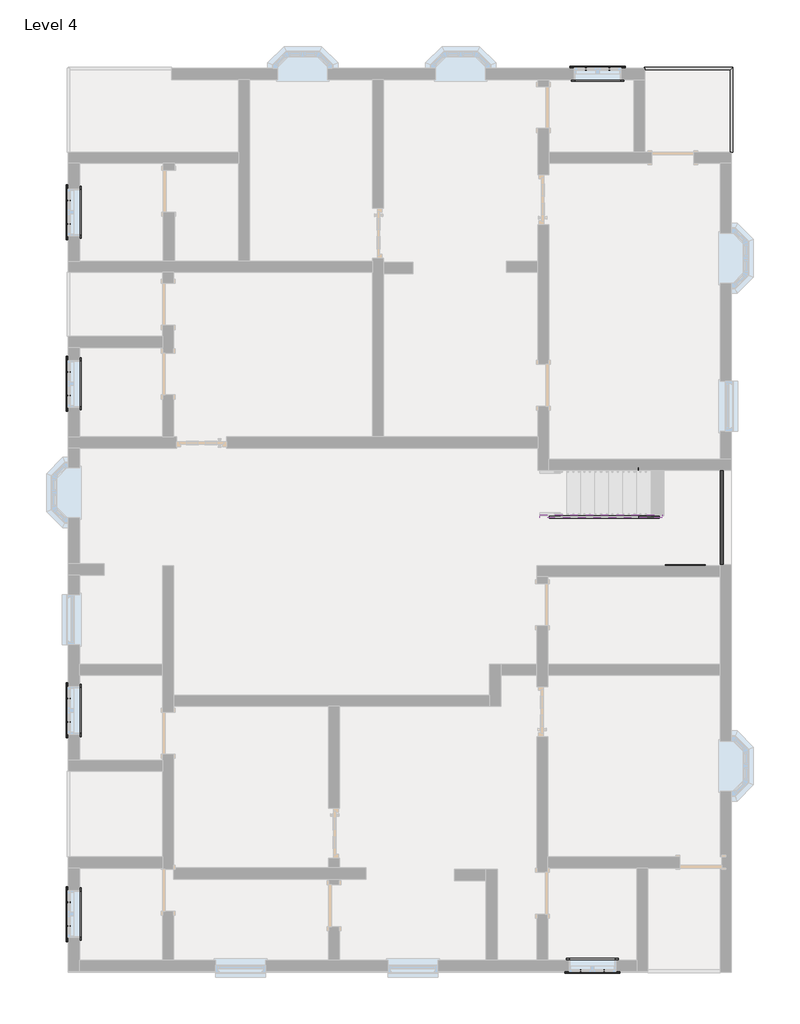
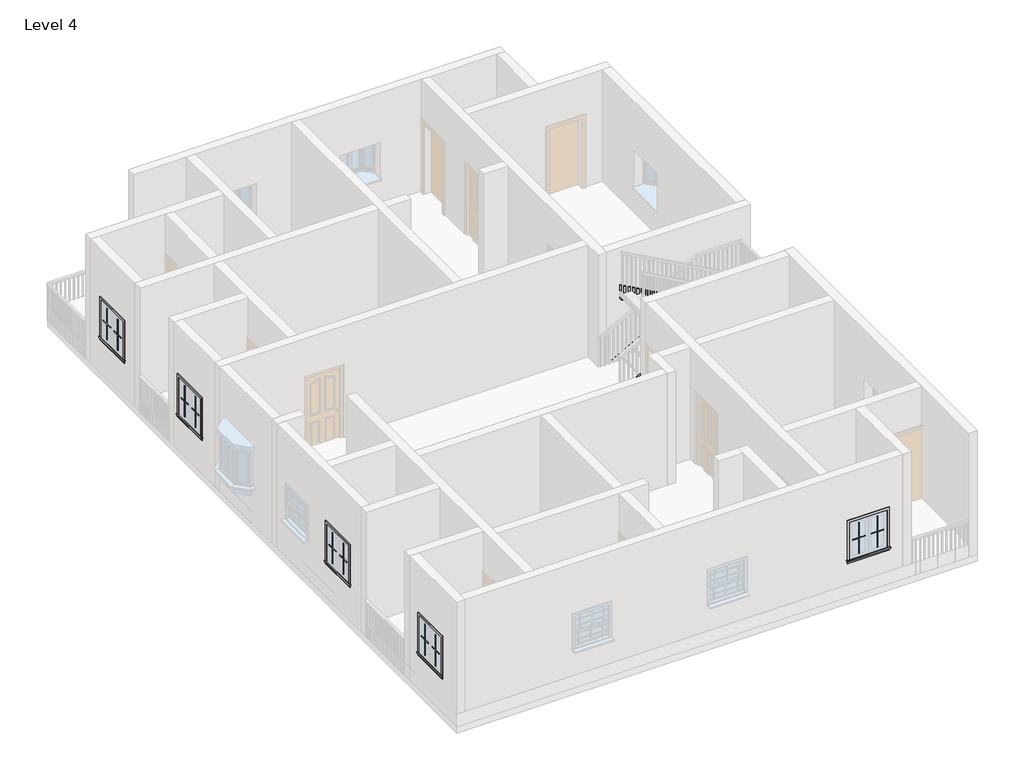
# One storey, part 4 of 4: 24 proxies, 5 members, 1 railing.
"""IFC4 building model written with IfcOpenShell, lengths in millimetres."""

from ifc_helpers import new_model, si_unit, frame, origin, place, context, project, spatial, polyline, outline, extrude, faceted_brep, transform, mapped, element, save
from components import muntin_pattern_2x2_muntin_pattern_2x2_b3fe6957, muntin_pattern_2x2_muntin_pattern_2x2_3e0ecaf2, trim_window_exterior_flat_with_sill_41619996, trim_window_interior_flat_picture_frame_51c85655

model = new_model("IFC4")

# Units and contexts
model_context = context("Model", 3, world=origin())
ifc_project = project(units=[si_unit("LENGTHUNIT", "METRE", prefix="MILLI")], contexts=[model_context])

# Site, building, storey
site = spatial("IfcSite", under=ifc_project)
building = spatial("IfcBuilding", under=site)
storey = spatial("IfcBuildingStorey", under=building, Name="Level 4", Elevation=9144.0)

# Proxies
placement = place(None, origin())
muntin_pattern_2x2_muntin_pattern_2x2_shape = muntin_pattern_2x2_muntin_pattern_2x2_b3fe6957(model_context)
element("IfcBuildingElementProxy", 1, Name="Muntin Pattern_2x2 : Muntin Pattern_2x2", ObjectType="Muntin Pattern_2x2 : Muntin Pattern_2x2", at=placement, inside=storey, context=model_context, shape_type="MappedRepresentation", body=[
    mapped(muntin_pattern_2x2_muntin_pattern_2x2_shape, transform((-7038.4808717, 5489.0318597, 10128.25), x_axis=(0.0, 1.0, 0.0), y_axis=(-1.0, 0.0, 0.0), z_axis=(0.0, 0.0, 1.0))),
])
element("IfcBuildingElementProxy", 2, Name="Muntin Pattern_2x2 : Muntin Pattern_2x2", ObjectType="Muntin Pattern_2x2 : Muntin Pattern_2x2", at=placement, inside=storey, context=model_context, shape_type="MappedRepresentation", body=[
    mapped(muntin_pattern_2x2_muntin_pattern_2x2_shape, transform((-7038.4808717, 2366.9422293, 10128.25), x_axis=(0.0, 1.0, 0.0), y_axis=(-1.0, 0.0, 0.0), z_axis=(0.0, 0.0, 1.0))),
])
element("IfcBuildingElementProxy", 3, Name="Muntin Pattern_2x2 : Muntin Pattern_2x2", ObjectType="Muntin Pattern_2x2 : Muntin Pattern_2x2", at=placement, inside=storey, context=model_context, shape_type="MappedRepresentation", body=[
    mapped(muntin_pattern_2x2_muntin_pattern_2x2_shape, transform((2376.9816283, 8312.1297293, 10128.25), x_axis=(1.0, 0.0, 0.0), y_axis=(0.0, 1.0, 0.0), z_axis=(0.0, 0.0, 1.0))),
])
element("IfcBuildingElementProxy", 4, Name="Muntin Pattern_2x2 : Muntin Pattern_2x2", ObjectType="Muntin Pattern_2x2 : Muntin Pattern_2x2", at=placement, inside=storey, context=model_context, shape_type="MappedRepresentation", body=[
    mapped(muntin_pattern_2x2_muntin_pattern_2x2_shape, transform((2710.3566283, -8102.6202707, 10128.25), x_axis=(-1.0, 0.0, 0.0), y_axis=(0.0, -1.0, 0.0), z_axis=(0.0, 0.0, 1.0))),
])
element("IfcBuildingElementProxy", 5, Name="Muntin Pattern_2x2 : Muntin Pattern_2x2", ObjectType="Muntin Pattern_2x2 : Muntin Pattern_2x2", at=placement, inside=storey, context=model_context, shape_type="MappedRepresentation", body=[
    mapped(muntin_pattern_2x2_muntin_pattern_2x2_shape, transform((-7038.4808717, -7285.0577707, 10128.25), x_axis=(0.0, 1.0, 0.0), y_axis=(-1.0, 0.0, 0.0), z_axis=(0.0, 0.0, 1.0))),
])
element("IfcBuildingElementProxy", 6, Name="Muntin Pattern_2x2 : Muntin Pattern_2x2", ObjectType="Muntin Pattern_2x2 : Muntin Pattern_2x2", at=placement, inside=storey, context=model_context, shape_type="MappedRepresentation", body=[
    mapped(muntin_pattern_2x2_muntin_pattern_2x2_shape, transform((-7038.4808717, -3576.6577707, 10128.25), x_axis=(0.0, 1.0, 0.0), y_axis=(-1.0, 0.0, 0.0), z_axis=(0.0, 0.0, 1.0))),
])
muntin_pattern_2x2_muntin_pattern_2x2_2_shape = muntin_pattern_2x2_muntin_pattern_2x2_3e0ecaf2(model_context)
element("IfcBuildingElementProxy", 7, Name="Muntin Pattern_2x2 : Muntin Pattern_2x2", ObjectType="Muntin Pattern_2x2 : Muntin Pattern_2x2", at=placement, inside=storey, context=model_context, shape_type="MappedRepresentation", body=[
    mapped(muntin_pattern_2x2_muntin_pattern_2x2_2_shape, transform((-7038.4808717, 5917.6568597, 10128.25), x_axis=(0.0, -1.0, 0.0), y_axis=(1.0, 0.0, 0.0), z_axis=(0.0, 0.0, 1.0))),
])
element("IfcBuildingElementProxy", 8, Name="Muntin Pattern_2x2 : Muntin Pattern_2x2", ObjectType="Muntin Pattern_2x2 : Muntin Pattern_2x2", at=placement, inside=storey, context=model_context, shape_type="MappedRepresentation", body=[
    mapped(muntin_pattern_2x2_muntin_pattern_2x2_2_shape, transform((-7038.4808717, 2795.5672293, 10128.25), x_axis=(0.0, -1.0, 0.0), y_axis=(1.0, 0.0, 0.0), z_axis=(0.0, 0.0, 1.0))),
])
element("IfcBuildingElementProxy", 9, Name="Muntin Pattern_2x2 : Muntin Pattern_2x2", ObjectType="Muntin Pattern_2x2 : Muntin Pattern_2x2", at=placement, inside=storey, context=model_context, shape_type="MappedRepresentation", body=[
    mapped(muntin_pattern_2x2_muntin_pattern_2x2_2_shape, transform((2805.6066283, 8312.1297293, 10128.25), x_axis=(-1.0, 0.0, 0.0), y_axis=(0.0, -1.0, 0.0), z_axis=(0.0, 0.0, 1.0))),
])
element("IfcBuildingElementProxy", 10, Name="Muntin Pattern_2x2 : Muntin Pattern_2x2", ObjectType="Muntin Pattern_2x2 : Muntin Pattern_2x2", at=placement, inside=storey, context=model_context, shape_type="MappedRepresentation", body=[
    mapped(muntin_pattern_2x2_muntin_pattern_2x2_2_shape, transform((2281.7316283, -8102.6202707, 10128.25), x_axis=(1.0, 0.0, 0.0), y_axis=(0.0, 1.0, 0.0), z_axis=(0.0, 0.0, 1.0))),
])
element("IfcBuildingElementProxy", 11, Name="Muntin Pattern_2x2 : Muntin Pattern_2x2", ObjectType="Muntin Pattern_2x2 : Muntin Pattern_2x2", at=placement, inside=storey, context=model_context, shape_type="MappedRepresentation", body=[
    mapped(muntin_pattern_2x2_muntin_pattern_2x2_2_shape, transform((-7038.4808717, -6856.4327707, 10128.25), x_axis=(0.0, -1.0, 0.0), y_axis=(1.0, 0.0, 0.0), z_axis=(0.0, 0.0, 1.0))),
])
element("IfcBuildingElementProxy", 12, Name="Muntin Pattern_2x2 : Muntin Pattern_2x2", ObjectType="Muntin Pattern_2x2 : Muntin Pattern_2x2", at=placement, inside=storey, context=model_context, shape_type="MappedRepresentation", body=[
    mapped(muntin_pattern_2x2_muntin_pattern_2x2_2_shape, transform((-7038.4808717, -3148.0327707, 10128.25), x_axis=(0.0, -1.0, 0.0), y_axis=(1.0, 0.0, 0.0), z_axis=(0.0, 0.0, 1.0))),
])
trim_window_exterior_flat_with_sill_shape = trim_window_exterior_flat_with_sill_41619996(model_context)
element("IfcBuildingElementProxy", 13, Name="Trim-Window-Exterior-Flat : with Sill", ObjectType="Trim-Window-Exterior-Flat : with Sill", at=placement, inside=storey, context=model_context, shape_type="MappedRepresentation", body=[
    mapped(trim_window_exterior_flat_with_sill_shape, transform((-7048.0058717, 5703.3443597, 10972.8), x_axis=(0.0, -1.0, 0.0), y_axis=(0.0, 0.0, 1.0), z_axis=(-1.0, 0.0, 0.0))),
])
element("IfcBuildingElementProxy", 14, Name="Trim-Window-Exterior-Flat : with Sill", ObjectType="Trim-Window-Exterior-Flat : with Sill", at=placement, inside=storey, context=model_context, shape_type="MappedRepresentation", body=[
    mapped(trim_window_exterior_flat_with_sill_shape, transform((-7048.0058717, 2581.2547293, 10972.8), x_axis=(0.0, -1.0, 0.0), y_axis=(0.0, 0.0, 1.0), z_axis=(-1.0, 0.0, 0.0))),
])
element("IfcBuildingElementProxy", 15, Name="Trim-Window-Exterior-Flat : with Sill", ObjectType="Trim-Window-Exterior-Flat : with Sill", at=placement, inside=storey, context=model_context, shape_type="MappedRepresentation", body=[
    mapped(trim_window_exterior_flat_with_sill_shape, transform((2591.2941283, 8321.6547293, 10972.8), x_axis=(-1.0, 0.0, 0.0), y_axis=(0.0, 0.0, 1.0), z_axis=(0.0, 1.0, 0.0))),
])
element("IfcBuildingElementProxy", 16, Name="Trim-Window-Exterior-Flat : with Sill", ObjectType="Trim-Window-Exterior-Flat : with Sill", at=placement, inside=storey, context=model_context, shape_type="MappedRepresentation", body=[
    mapped(trim_window_exterior_flat_with_sill_shape, transform((2496.0441283, -8112.1452707, 10972.8), x_axis=(1.0, 0.0, 0.0), y_axis=(0.0, 0.0, 1.0), z_axis=(0.0, -1.0, 0.0))),
])
element("IfcBuildingElementProxy", 17, Name="Trim-Window-Exterior-Flat : with Sill", ObjectType="Trim-Window-Exterior-Flat : with Sill", at=placement, inside=storey, context=model_context, shape_type="MappedRepresentation", body=[
    mapped(trim_window_exterior_flat_with_sill_shape, transform((-7048.0058717, -7070.7452707, 10972.8), x_axis=(0.0, -1.0, 0.0), y_axis=(0.0, 0.0, 1.0), z_axis=(-1.0, 0.0, 0.0))),
])
element("IfcBuildingElementProxy", 18, Name="Trim-Window-Exterior-Flat : with Sill", ObjectType="Trim-Window-Exterior-Flat : with Sill", at=placement, inside=storey, context=model_context, shape_type="MappedRepresentation", body=[
    mapped(trim_window_exterior_flat_with_sill_shape, transform((-7048.0058717, -3362.3452707, 10972.8), x_axis=(0.0, -1.0, 0.0), y_axis=(0.0, 0.0, 1.0), z_axis=(-1.0, 0.0, 0.0))),
])
trim_window_interior_flat_picture_frame_shape = trim_window_interior_flat_picture_frame_51c85655(model_context)
element("IfcBuildingElementProxy", 19, Name="Trim-Window-Interior-Flat : Picture Frame", ObjectType="Trim-Window-Interior-Flat : Picture Frame", at=placement, inside=storey, context=model_context, shape_type="MappedRepresentation", body=[
    mapped(trim_window_interior_flat_picture_frame_shape, transform((-6844.8058717, 5703.3443597, 10972.8), x_axis=(0.0, 1.0, 0.0), y_axis=(0.0, 0.0, 1.0), z_axis=(1.0, 0.0, 0.0))),
])
element("IfcBuildingElementProxy", 20, Name="Trim-Window-Interior-Flat : Picture Frame", ObjectType="Trim-Window-Interior-Flat : Picture Frame", at=placement, inside=storey, context=model_context, shape_type="MappedRepresentation", body=[
    mapped(trim_window_interior_flat_picture_frame_shape, transform((-6844.8058717, 2581.2547293, 10972.8), x_axis=(0.0, 1.0, 0.0), y_axis=(0.0, 0.0, 1.0), z_axis=(1.0, 0.0, 0.0))),
])
element("IfcBuildingElementProxy", 21, Name="Trim-Window-Interior-Flat : Picture Frame", ObjectType="Trim-Window-Interior-Flat : Picture Frame", at=placement, inside=storey, context=model_context, shape_type="MappedRepresentation", body=[
    mapped(trim_window_interior_flat_picture_frame_shape, transform((2591.2941283, 8118.4547293, 10972.8), x_axis=(1.0, 0.0, 0.0), y_axis=(0.0, 0.0, 1.0), z_axis=(0.0, -1.0, 0.0))),
])
element("IfcBuildingElementProxy", 22, Name="Trim-Window-Interior-Flat : Picture Frame", ObjectType="Trim-Window-Interior-Flat : Picture Frame", at=placement, inside=storey, context=model_context, shape_type="MappedRepresentation", body=[
    mapped(trim_window_interior_flat_picture_frame_shape, transform((2496.0441283, -7908.9452707, 10972.8), x_axis=(-1.0, 0.0, 0.0), y_axis=(0.0, 0.0, 1.0), z_axis=(0.0, 1.0, 0.0))),
])
element("IfcBuildingElementProxy", 23, Name="Trim-Window-Interior-Flat : Picture Frame", ObjectType="Trim-Window-Interior-Flat : Picture Frame", at=placement, inside=storey, context=model_context, shape_type="MappedRepresentation", body=[
    mapped(trim_window_interior_flat_picture_frame_shape, transform((-6844.8058717, -7070.7452707, 10972.8), x_axis=(0.0, 1.0, 0.0), y_axis=(0.0, 0.0, 1.0), z_axis=(1.0, 0.0, 0.0))),
])
element("IfcBuildingElementProxy", 24, Name="Trim-Window-Interior-Flat : Picture Frame", ObjectType="Trim-Window-Interior-Flat : Picture Frame", at=placement, inside=storey, context=model_context, shape_type="MappedRepresentation", body=[
    mapped(trim_window_interior_flat_picture_frame_shape, transform((-6844.8058717, -3362.3452707, 10972.8), x_axis=(0.0, 1.0, 0.0), y_axis=(0.0, 0.0, 1.0), z_axis=(1.0, 0.0, 0.0))),
])

# Members
element("IfcMember", 25, ObjectType="Stringer - 2\" Width", at=placement, inside=storey, context=model_context, shape_type="SweptSolid", body=[
    extrude(outline(polyline([(9354.6757607, 1537.1941283), (9144.0, 1537.1941283), (9144.0, 1786.1766781), (10591.8, 4407.1563102), (10591.8, 3776.7834593), (9354.6757607, 1537.1941283)])), frame((0.0, 1006.4547293, 0.0), z_axis=(0.0, 1.0, 0.0), x_axis=(0.0, 0.0, 1.0)), (0.0, 0.0, 1.0), 50.8),
])
element("IfcMember", 26, ObjectType="Stringer - 2\" Width", at=placement, inside=storey, context=model_context, shape_type="SweptSolid", body=[
    extrude(outline(polyline([(4826.4941283, 1057.2547293), (4877.2941283, 1057.2547293), (4877.2941283, -714.2964201), (4826.4941283, -714.2964201), (4826.4941283, 1057.2547293)])), frame((0.0, 0.0, 10287.0), z_axis=(0.0, 0.0, 1.0), x_axis=(1.0, 0.0, 0.0)), (0.0, 0.0, 1.0), 304.8),
])
element("IfcMember", 27, ObjectType="Stringer - 2\" Width", at=placement, inside=storey, context=model_context, shape_type="SweptSolid", body=[
    extrude(outline(polyline([(10287.0, 4555.0346706), (11954.0215532, 1537.1941283), (11605.8106009, 1537.1941283), (10287.0, 3924.6618197), (10287.0, 4555.0346706)])), frame((0.0, -765.0964201, 0.0), z_axis=(0.0, 1.0, 0.0), x_axis=(0.0, 0.0, 1.0)), (0.0, 0.0, 1.0), 50.8),
])
element("IfcMember", 28, ObjectType="Stringer - 2\" Width", at=placement, inside=storey, context=model_context, shape_type="SweptSolid", body=[
    extrude(outline(polyline([(9354.6757607, 1537.1941283), (9144.0, 1537.1941283), (9144.0, 1786.1766781), (10209.4963497, 3715.0648053), (10557.7073019, 3715.0648053), (9354.6757607, 1537.1941283)])), frame((0.0, 130.1547293, 0.0), z_axis=(0.0, 1.0, 0.0), x_axis=(0.0, 0.0, 1.0)), (0.0, 0.0, 1.0), 50.8),
])
element("IfcMember", 29, ObjectType="Stringer - 2\" Width", at=placement, inside=storey, context=model_context, shape_type="SweptSolid", body=[
    extrude(outline(polyline([(10374.7177047, 3765.8648053), (10722.928657, 3765.8648053), (11954.0215532, 1537.1941283), (11605.8106009, 1537.1941283), (10374.7177047, 3765.8648053)])), frame((0.0, 142.8547293, 0.0), z_axis=(0.0, 1.0, 0.0), x_axis=(0.0, 0.0, 1.0)), (0.0, 0.0, 1.0), 50.8),
])

# Railing
element("IfcRailing", 30, ObjectType="Handrail - Rectangular", at=placement, inside=storey, context=model_context, shape_type="SolidModel", body=[
    faceted_brep([(3442.1941283, 8347.0547293, 10058.4), (3442.1941283, 8347.0547293, 10007.6), (3442.1941283, 8296.2547293, 10007.6), (3442.1941283, 8296.2547293, 10058.4), (5055.0941283, 8347.0547293, 10058.4), (5055.0941283, 8347.0547293, 10007.6), (5004.2941283, 8296.2547293, 10007.6), (5004.2941283, 8296.2547293, 10058.4), (5055.0941283, 6797.6547293, 10058.4), (5004.2941283, 6797.6547293, 10058.4), (5004.2941283, 6797.6547293, 10007.6), (5055.0941283, 6797.6547293, 10007.6)], [[[0, 1, 2, 3]], [[1, 0, 4, 5]], [[2, 1, 5, 6]], [[3, 2, 6, 7]], [[0, 3, 7, 4]], [[8, 9, 10, 11]], [[5, 4, 8, 11]], [[6, 5, 11, 10]], [[7, 6, 10, 9]], [[4, 7, 9, 8]]]),
    extrude(outline(polyline([(5020.1691283, 6908.7797293), (5039.2191283, 6908.7797293), (5039.2191283, 6889.7297293), (5020.1691283, 6889.7297293), (5020.1691283, 6908.7797293)])), frame((0.0, 0.0, 9144.0), z_axis=(0.0, 0.0, 1.0), x_axis=(1.0, 0.0, 0.0)), (0.0, 0.0, 1.0), 863.6),
    extrude(outline(polyline([(5020.1691283, 7010.3797293), (5039.2191283, 7010.3797293), (5039.2191283, 6991.3297293), (5020.1691283, 6991.3297293), (5020.1691283, 7010.3797293)])), frame((0.0, 0.0, 9144.0), z_axis=(0.0, 0.0, 1.0), x_axis=(1.0, 0.0, 0.0)), (0.0, 0.0, 1.0), 863.6),
    extrude(outline(polyline([(5020.1691283, 7111.9797293), (5039.2191283, 7111.9797293), (5039.2191283, 7092.9297293), (5020.1691283, 7092.9297293), (5020.1691283, 7111.9797293)])), frame((0.0, 0.0, 9144.0), z_axis=(0.0, 0.0, 1.0), x_axis=(1.0, 0.0, 0.0)), (0.0, 0.0, 1.0), 863.6),
    extrude(outline(polyline([(5020.1691283, 7213.5797293), (5039.2191283, 7213.5797293), (5039.2191283, 7194.5297293), (5020.1691283, 7194.5297293), (5020.1691283, 7213.5797293)])), frame((0.0, 0.0, 9144.0), z_axis=(0.0, 0.0, 1.0), x_axis=(1.0, 0.0, 0.0)), (0.0, 0.0, 1.0), 863.6),
    extrude(outline(polyline([(5020.1691283, 7315.1797293), (5039.2191283, 7315.1797293), (5039.2191283, 7296.1297293), (5020.1691283, 7296.1297293), (5020.1691283, 7315.1797293)])), frame((0.0, 0.0, 9144.0), z_axis=(0.0, 0.0, 1.0), x_axis=(1.0, 0.0, 0.0)), (0.0, 0.0, 1.0), 863.6),
    extrude(outline(polyline([(5020.1691283, 7416.7797293), (5039.2191283, 7416.7797293), (5039.2191283, 7397.7297293), (5020.1691283, 7397.7297293), (5020.1691283, 7416.7797293)])), frame((0.0, 0.0, 9144.0), z_axis=(0.0, 0.0, 1.0), x_axis=(1.0, 0.0, 0.0)), (0.0, 0.0, 1.0), 863.6),
    extrude(outline(polyline([(5020.1691283, 7518.3797293), (5039.2191283, 7518.3797293), (5039.2191283, 7499.3297293), (5020.1691283, 7499.3297293), (5020.1691283, 7518.3797293)])), frame((0.0, 0.0, 9144.0), z_axis=(0.0, 0.0, 1.0), x_axis=(1.0, 0.0, 0.0)), (0.0, 0.0, 1.0), 863.6),
    extrude(outline(polyline([(5020.1691283, 7619.9797293), (5039.2191283, 7619.9797293), (5039.2191283, 7600.9297293), (5020.1691283, 7600.9297293), (5020.1691283, 7619.9797293)])), frame((0.0, 0.0, 9144.0), z_axis=(0.0, 0.0, 1.0), x_axis=(1.0, 0.0, 0.0)), (0.0, 0.0, 1.0), 863.6),
    extrude(outline(polyline([(5020.1691283, 7721.5797293), (5039.2191283, 7721.5797293), (5039.2191283, 7702.5297293), (5020.1691283, 7702.5297293), (5020.1691283, 7721.5797293)])), frame((0.0, 0.0, 9144.0), z_axis=(0.0, 0.0, 1.0), x_axis=(1.0, 0.0, 0.0)), (0.0, 0.0, 1.0), 863.6),
    extrude(outline(polyline([(5020.1691283, 7823.1797293), (5039.2191283, 7823.1797293), (5039.2191283, 7804.1297293), (5020.1691283, 7804.1297293), (5020.1691283, 7823.1797293)])), frame((0.0, 0.0, 9144.0), z_axis=(0.0, 0.0, 1.0), x_axis=(1.0, 0.0, 0.0)), (0.0, 0.0, 1.0), 863.6),
    extrude(outline(polyline([(5020.1691283, 7924.7797293), (5039.2191283, 7924.7797293), (5039.2191283, 7905.7297293), (5020.1691283, 7905.7297293), (5020.1691283, 7924.7797293)])), frame((0.0, 0.0, 9144.0), z_axis=(0.0, 0.0, 1.0), x_axis=(1.0, 0.0, 0.0)), (0.0, 0.0, 1.0), 863.6),
    extrude(outline(polyline([(5020.1691283, 8026.3797293), (5039.2191283, 8026.3797293), (5039.2191283, 8007.3297293), (5020.1691283, 8007.3297293), (5020.1691283, 8026.3797293)])), frame((0.0, 0.0, 9144.0), z_axis=(0.0, 0.0, 1.0), x_axis=(1.0, 0.0, 0.0)), (0.0, 0.0, 1.0), 863.6),
    extrude(outline(polyline([(5020.1691283, 8127.9797293), (5039.2191283, 8127.9797293), (5039.2191283, 8108.9297293), (5020.1691283, 8108.9297293), (5020.1691283, 8127.9797293)])), frame((0.0, 0.0, 9144.0), z_axis=(0.0, 0.0, 1.0), x_axis=(1.0, 0.0, 0.0)), (0.0, 0.0, 1.0), 863.6),
    extrude(outline(polyline([(5020.1691283, 8229.5797293), (5039.2191283, 8229.5797293), (5039.2191283, 8210.5297293), (5020.1691283, 8210.5297293), (5020.1691283, 8229.5797293)])), frame((0.0, 0.0, 9144.0), z_axis=(0.0, 0.0, 1.0), x_axis=(1.0, 0.0, 0.0)), (0.0, 0.0, 1.0), 863.6),
    extrude(outline(polyline([(4956.6691283, 8312.1297293), (4956.6691283, 8331.1797293), (4975.7191283, 8331.1797293), (4975.7191283, 8312.1297293), (4956.6691283, 8312.1297293)])), frame((0.0, 0.0, 9144.0), z_axis=(0.0, 0.0, 1.0), x_axis=(1.0, 0.0, 0.0)), (0.0, 0.0, 1.0), 863.6),
    extrude(outline(polyline([(4855.0691283, 8312.1297293), (4855.0691283, 8331.1797293), (4874.1191283, 8331.1797293), (4874.1191283, 8312.1297293), (4855.0691283, 8312.1297293)])), frame((0.0, 0.0, 9144.0), z_axis=(0.0, 0.0, 1.0), x_axis=(1.0, 0.0, 0.0)), (0.0, 0.0, 1.0), 863.6),
    extrude(outline(polyline([(4753.4691283, 8312.1297293), (4753.4691283, 8331.1797293), (4772.5191283, 8331.1797293), (4772.5191283, 8312.1297293), (4753.4691283, 8312.1297293)])), frame((0.0, 0.0, 9144.0), z_axis=(0.0, 0.0, 1.0), x_axis=(1.0, 0.0, 0.0)), (0.0, 0.0, 1.0), 863.6),
    extrude(outline(polyline([(4651.8691283, 8312.1297293), (4651.8691283, 8331.1797293), (4670.9191283, 8331.1797293), (4670.9191283, 8312.1297293), (4651.8691283, 8312.1297293)])), frame((0.0, 0.0, 9144.0), z_axis=(0.0, 0.0, 1.0), x_axis=(1.0, 0.0, 0.0)), (0.0, 0.0, 1.0), 863.6),
    extrude(outline(polyline([(4550.2691283, 8312.1297293), (4550.2691283, 8331.1797293), (4569.3191283, 8331.1797293), (4569.3191283, 8312.1297293), (4550.2691283, 8312.1297293)])), frame((0.0, 0.0, 9144.0), z_axis=(0.0, 0.0, 1.0), x_axis=(1.0, 0.0, 0.0)), (0.0, 0.0, 1.0), 863.6),
    extrude(outline(polyline([(4448.6691283, 8312.1297293), (4448.6691283, 8331.1797293), (4467.7191283, 8331.1797293), (4467.7191283, 8312.1297293), (4448.6691283, 8312.1297293)])), frame((0.0, 0.0, 9144.0), z_axis=(0.0, 0.0, 1.0), x_axis=(1.0, 0.0, 0.0)), (0.0, 0.0, 1.0), 863.6),
    extrude(outline(polyline([(4347.0691283, 8312.1297293), (4347.0691283, 8331.1797293), (4366.1191283, 8331.1797293), (4366.1191283, 8312.1297293), (4347.0691283, 8312.1297293)])), frame((0.0, 0.0, 9144.0), z_axis=(0.0, 0.0, 1.0), x_axis=(1.0, 0.0, 0.0)), (0.0, 0.0, 1.0), 863.6),
    extrude(outline(polyline([(4245.4691283, 8312.1297293), (4245.4691283, 8331.1797293), (4264.5191283, 8331.1797293), (4264.5191283, 8312.1297293), (4245.4691283, 8312.1297293)])), frame((0.0, 0.0, 9144.0), z_axis=(0.0, 0.0, 1.0), x_axis=(1.0, 0.0, 0.0)), (0.0, 0.0, 1.0), 863.6),
    extrude(outline(polyline([(4143.8691283, 8312.1297293), (4143.8691283, 8331.1797293), (4162.9191283, 8331.1797293), (4162.9191283, 8312.1297293), (4143.8691283, 8312.1297293)])), frame((0.0, 0.0, 9144.0), z_axis=(0.0, 0.0, 1.0), x_axis=(1.0, 0.0, 0.0)), (0.0, 0.0, 1.0), 863.6),
    extrude(outline(polyline([(4042.2691283, 8312.1297293), (4042.2691283, 8331.1797293), (4061.3191283, 8331.1797293), (4061.3191283, 8312.1297293), (4042.2691283, 8312.1297293)])), frame((0.0, 0.0, 9144.0), z_axis=(0.0, 0.0, 1.0), x_axis=(1.0, 0.0, 0.0)), (0.0, 0.0, 1.0), 863.6),
    extrude(outline(polyline([(3940.6691283, 8312.1297293), (3940.6691283, 8331.1797293), (3959.7191283, 8331.1797293), (3959.7191283, 8312.1297293), (3940.6691283, 8312.1297293)])), frame((0.0, 0.0, 9144.0), z_axis=(0.0, 0.0, 1.0), x_axis=(1.0, 0.0, 0.0)), (0.0, 0.0, 1.0), 863.6),
    extrude(outline(polyline([(3839.0691283, 8312.1297293), (3839.0691283, 8331.1797293), (3858.1191283, 8331.1797293), (3858.1191283, 8312.1297293), (3839.0691283, 8312.1297293)])), frame((0.0, 0.0, 9144.0), z_axis=(0.0, 0.0, 1.0), x_axis=(1.0, 0.0, 0.0)), (0.0, 0.0, 1.0), 863.6),
    extrude(outline(polyline([(3737.4691283, 8312.1297293), (3737.4691283, 8331.1797293), (3756.5191283, 8331.1797293), (3756.5191283, 8312.1297293), (3737.4691283, 8312.1297293)])), frame((0.0, 0.0, 9144.0), z_axis=(0.0, 0.0, 1.0), x_axis=(1.0, 0.0, 0.0)), (0.0, 0.0, 1.0), 863.6),
    extrude(outline(polyline([(3635.8691283, 8312.1297293), (3635.8691283, 8331.1797293), (3654.9191283, 8331.1797293), (3654.9191283, 8312.1297293), (3635.8691283, 8312.1297293)])), frame((0.0, 0.0, 9144.0), z_axis=(0.0, 0.0, 1.0), x_axis=(1.0, 0.0, 0.0)), (0.0, 0.0, 1.0), 863.6),
    extrude(outline(polyline([(3534.2691283, 8312.1297293), (3534.2691283, 8331.1797293), (3553.3191283, 8331.1797293), (3553.3191283, 8312.1297293), (3534.2691283, 8312.1297293)])), frame((0.0, 0.0, 9144.0), z_axis=(0.0, 0.0, 1.0), x_axis=(1.0, 0.0, 0.0)), (0.0, 0.0, 1.0), 863.6),
    extrude(outline(polyline([(5020.1691283, 8312.1297293), (5020.1691283, 8331.1797293), (5039.2191283, 8331.1797293), (5039.2191283, 8312.1297293), (5020.1691283, 8312.1297293)])), frame((0.0, 0.0, 9144.0), z_axis=(0.0, 0.0, 1.0), x_axis=(1.0, 0.0, 0.0)), (0.0, 0.0, 1.0), 863.6),
    extrude(outline(polyline([(5020.1691283, 6816.7047293), (5039.2191283, 6816.7047293), (5039.2191283, 6797.6547293), (5020.1691283, 6797.6547293), (5020.1691283, 6816.7047293)])), frame((0.0, 0.0, 9144.0), z_axis=(0.0, 0.0, 1.0), x_axis=(1.0, 0.0, 0.0)), (0.0, 0.0, 1.0), 863.6),
    extrude(outline(polyline([(3442.1941283, 8312.1297293), (3442.1941283, 8331.1797293), (3461.2441283, 8331.1797293), (3461.2441283, 8312.1297293), (3442.1941283, 8312.1297293)])), frame((0.0, 0.0, 9144.0), z_axis=(0.0, 0.0, 1.0), x_axis=(1.0, 0.0, 0.0)), (0.0, 0.0, 1.0), 863.6),
])

save(model, "model.ifc")

# Revit data of these elements
# Type "Muntin Pattern_2x2 : Muntin Pattern_2x2"
#   Width [instance default] = 4' - 0"
#   Thickness = 0' - 0 1/2"
#   Height [instance default] = 4' - 0"
#   Distance = 0' - 0 3/4"
#   Interior Material [instance default] = none
#   Exterior Material [instance default] = none
#   Default Elevation = 0
# Type "Trim-Window-Exterior-Flat : with Sill"
#   Trim Width = 0' - 2 1/4"
#   Trim Thickness_Picture Frame = 0' - 1 1/4"
#   Trim Thickness_with Sill = 0' - 0 3/4"
#   Sill Thickness = 0' - 1 1/4"
#   Opening Width [instance default] = 2' - 0"
#   Opening Height [instance default] = 3' - 0"
#   Default Elevation = 4' - 0"
#   Sill = yes
#   Picture Frame = no
#   Trim Material [instance default] = none
# Type "Trim-Window-Interior-Flat : Picture Frame"
#   Trim Thickness_Picture Frame = 0' - 1 1/4"
#   Trim Width = 0' - 2 1/4"
#   Trim Thickness_with Sill = 0' - 0 3/4"
#   Sill Thickness = 0' - 1 1/4"
#   Opening Width [instance default] = 2' - 0"
#   Opening Height [instance default] = 3' - 0"
#   Default Elevation = 4' - 0"
#   Sill = no
#   Picture Frame = yes
#   Trim Material [instance default] = none
# Type "Handrail - Rectangular"
#   Assembly Code = "C2010400"
#   built-in parameter 1008612 = 0.0416667 (stored number, unit not read)
#   built-in parameter 1008611 = 0.0416667 (stored number, unit not read)
#   built-in parameter 1008609 = 0.333333 (stored number, unit not read)
#   built-in parameter 1008604 = 0.166667 (stored number, unit not read)
#   built-in parameter 1008603 = 0.166667 (stored number, unit not read)
#   Railing Height = 3' - 0"
#   built-in parameter 1008630 = 2
#   built-in parameter 1008610 = 2
#   built-in parameter 1008618 = Baluster - Square : 3/4"
# Elements 1, 2, 3, 4, 5, 6, 7, 8, 9, 10, 11, 12 (IfcBuildingElementProxy, "Muntin Pattern_2x2 : Muntin Pattern_2x2")
#   Width = 0' - 11 5/8"
#   Height = 2' - 6 1/2"
#   Interior Material = Wood - Stained
#   Exterior Material = Clad - White
#   Phase Created = New Construction
#   Materials on its faces: "Clad - White", "Wood - Stained"
# Elements 13, 14, 15, 16, 17, 18 (IfcBuildingElementProxy, "Trim-Window-Exterior-Flat : with Sill")
#   Opening Width = 2' - 10"
#   Opening Height = 3' - 0"
#   Trim Material = Clad - White
#   Phase Created = New Construction
#   Materials on its faces: "Clad - White"
# Elements 19, 20, 21, 22, 23, 24 (IfcBuildingElementProxy, "Trim-Window-Interior-Flat : Picture Frame")
#   Opening Width = 2' - 10"
#   Opening Height = 3' - 0"
#   Trim Material = Wood - Stained
#   Phase Created = New Construction
#   Materials on its faces: "Wood - Stained"
# Elements 25, 27, 28, 29 (IfcMember, "Stringer - 2\" Width")
#   Phase Created = New Construction
# Element 26 (IfcMember, "Stringer - 2\" Width")
#   Phase Created = New Construction
#   Materials on its faces: "Render Material 41-165-0"
# Element 30 (IfcRailing, "Handrail - Rectangular")
#   Phase Created = New Construction
# Materials
#   "Clad - White": class "Wood", colour RGB 242 242 238, transparency 0, Cost = 0
#   "Wood - Stained": class "Wood", colour RGB 224 178 126, transparency 0, Cost = 0
#   "Render Material 41-165-0": colour RGB 41 165 0, transparency 0
